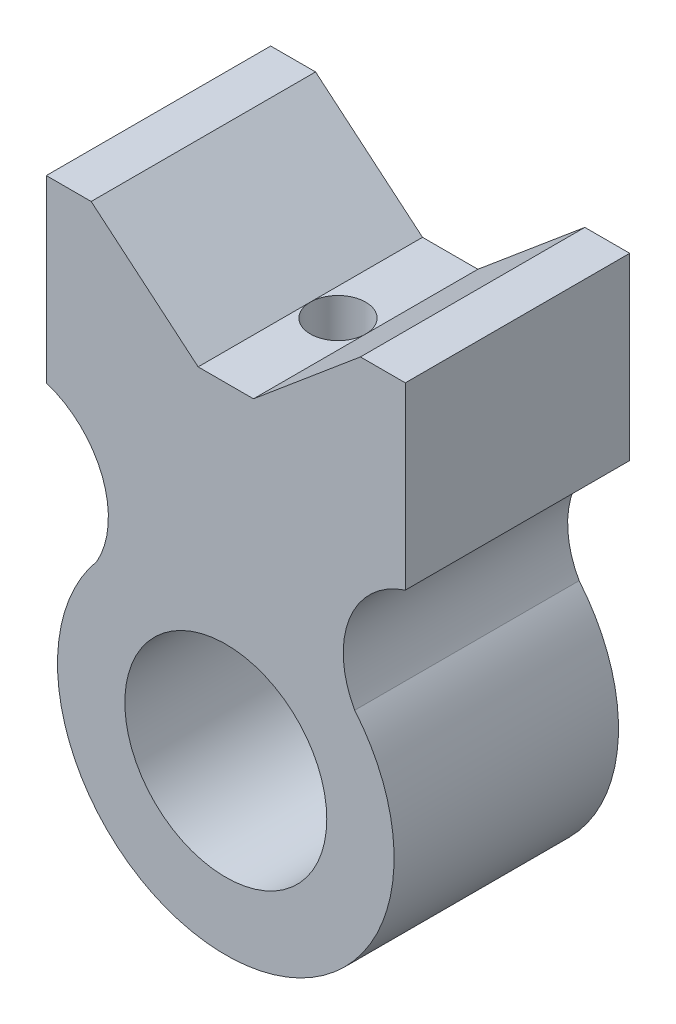
ISO-10303-21;
HEADER;
FILE_DESCRIPTION(('STEP AP214'),'2;1');
FILE_NAME('part.step','',(''),(''),'','','');
FILE_SCHEMA(('AUTOMOTIVE_DESIGN { 1 0 10303 214 1 1 1 1 }'));
ENDSEC;
DATA;
#1=APPLICATION_CONTEXT('core data for automotive mechanical design processes');
#2=APPLICATION_PROTOCOL_DEFINITION('international standard','automotive_design',2000,#1);
#3=PRODUCT_CONTEXT('',#1,'mechanical');
#4=PRODUCT('Part','Part','',(#3));
#5=PRODUCT_RELATED_PRODUCT_CATEGORY('part','',(#4));
#6=PRODUCT_DEFINITION_FORMATION('','',#4);
#7=PRODUCT_DEFINITION_CONTEXT('part definition',#1,'design');
#8=PRODUCT_DEFINITION('design','',#6,#7);
#9=PRODUCT_DEFINITION_SHAPE('','',#8);
#10=(LENGTH_UNIT() NAMED_UNIT(*) SI_UNIT(.MILLI.,.METRE.));
#11=(NAMED_UNIT(*) PLANE_ANGLE_UNIT() SI_UNIT($,.RADIAN.));
#12=(NAMED_UNIT(*) SI_UNIT($,.STERADIAN.) SOLID_ANGLE_UNIT());
#13=UNCERTAINTY_MEASURE_WITH_UNIT(LENGTH_MEASURE(1.E-05),#10,'distance_accuracy_value','');
#14=(GEOMETRIC_REPRESENTATION_CONTEXT(3) GLOBAL_UNCERTAINTY_ASSIGNED_CONTEXT((#13)) GLOBAL_UNIT_ASSIGNED_CONTEXT((#10,
#11,#12)) REPRESENTATION_CONTEXT('',''));
#15=CARTESIAN_POINT('',(0.,0.,0.));
#16=DIRECTION('',(0.,0.,1.));
#17=DIRECTION('',(1.,0.,0.));
#18=AXIS2_PLACEMENT_3D('',#15,#16,#17);
#19=CARTESIAN_POINT('',(46.1646162627975,33.8983044104148,25.));
#20=DIRECTION('',(0.,0.,-1.));
#21=DIRECTION('',(-1.,0.,0.));
#22=AXIS2_PLACEMENT_3D('',#19,#20,#21);
#23=PLANE('',#22);
#24=CARTESIAN_POINT('',(46.1646162627975,33.8983044104148,25.));
#25=DIRECTION('',(0.,0.,-1.));
#26=DIRECTION('',(-1.,0.,0.));
#27=AXIS2_PLACEMENT_3D('',#24,#25,#26);
#28=CIRCLE('',#27,20.);
#29=CARTESIAN_POINT('',(28.7266666169617,24.1045353632452,25.));
#30=VERTEX_POINT('',#29);
#31=CARTESIAN_POINT('',(39.9999281481161,52.9245131880117,25.));
#32=VERTEX_POINT('',#31);
#33=EDGE_CURVE('E185',#30,#32,#28,.T.);
#34=ORIENTED_EDGE('',*,*,#33,.T.);
#35=DIRECTION('',(0.,1.,0.));
#36=VECTOR('',#35,1.);
#37=CARTESIAN_POINT('',(39.9999281481161,92.9245131880117,25.));
#38=LINE('',#37,#36);
#39=CARTESIAN_POINT('',(39.9999281481161,92.9245131880117,25.));
#40=VERTEX_POINT('',#39);
#41=EDGE_CURVE('E111',#32,#40,#38,.T.);
#42=ORIENTED_EDGE('',*,*,#41,.T.);
#43=DIRECTION('',(-1.,0.,0.));
#44=VECTOR('',#43,1.);
#45=CARTESIAN_POINT('',(29.9999281481161,92.9245131880117,25.));
#46=LINE('',#45,#44);
#47=CARTESIAN_POINT('',(29.9999281481161,92.9245131880117,25.));
#48=VERTEX_POINT('',#47);
#49=EDGE_CURVE('E202',#40,#48,#46,.T.);
#50=ORIENTED_EDGE('',*,*,#49,.T.);
#51=DIRECTION('',(-0.766044443118979,-0.642787609686538,0.));
#52=VECTOR('',#51,1.);
#53=CARTESIAN_POINT('',(6.16485629623179,72.9245131880117,25.));
#54=LINE('',#53,#52);
#55=CARTESIAN_POINT('',(6.16485629623179,72.9245131880117,25.));
#56=VERTEX_POINT('',#55);
#57=EDGE_CURVE('E217',#48,#56,#54,.T.);
#58=ORIENTED_EDGE('',*,*,#57,.T.);
#59=DIRECTION('',(-1.,0.,0.));
#60=VECTOR('',#59,1.);
#61=CARTESIAN_POINT('',(-6.165,72.9245131880117,25.));
#62=LINE('',#61,#60);
#63=CARTESIAN_POINT('',(-6.165,72.9245131880117,25.));
#64=VERTEX_POINT('',#63);
#65=EDGE_CURVE('E219',#56,#64,#62,.T.);
#66=ORIENTED_EDGE('',*,*,#65,.T.);
#67=DIRECTION('',(-0.766044443118974,0.642787609686544,0.));
#68=VECTOR('',#67,1.);
#69=CARTESIAN_POINT('',(-30.0000718518839,92.9245131880117,25.));
#70=LINE('',#69,#68);
#71=CARTESIAN_POINT('',(-30.0000718518839,92.9245131880117,25.));
#72=VERTEX_POINT('',#71);
#73=EDGE_CURVE('E225',#64,#72,#70,.T.);
#74=ORIENTED_EDGE('',*,*,#73,.T.);
#75=DIRECTION('',(-1.,0.,0.));
#76=VECTOR('',#75,1.);
#77=CARTESIAN_POINT('',(-40.0000718518839,92.9245131880117,25.));
#78=LINE('',#77,#76);
#79=CARTESIAN_POINT('',(-40.0000718518839,92.9245131880117,25.));
#80=VERTEX_POINT('',#79);
#81=EDGE_CURVE('E140',#72,#80,#78,.T.);
#82=ORIENTED_EDGE('',*,*,#81,.T.);
#83=DIRECTION('',(0.,-1.,0.));
#84=VECTOR('',#83,1.);
#85=CARTESIAN_POINT('',(-40.0000718518839,52.9245131880117,25.));
#86=LINE('',#85,#84);
#87=CARTESIAN_POINT('',(-40.0000718518839,52.9245131880117,25.));
#88=VERTEX_POINT('',#87);
#89=EDGE_CURVE('E132',#80,#88,#86,.T.);
#90=ORIENTED_EDGE('',*,*,#89,.T.);
#91=CARTESIAN_POINT('',(-46.1646383870159,33.8982650178145,25.));
#92=DIRECTION('',(0.,0.,-1.));
#93=DIRECTION('',(1.,0.,0.));
#94=AXIS2_PLACEMENT_3D('',#91,#92,#93);
#95=CIRCLE('',#94,20.);
#96=CARTESIAN_POINT('',(-28.7266666169617,24.1045353632452,25.));
#97=VERTEX_POINT('',#96);
#98=EDGE_CURVE('E137',#88,#97,#95,.T.);
#99=ORIENTED_EDGE('',*,*,#98,.T.);
#100=CARTESIAN_POINT('',(0.,0.,25.));
#101=DIRECTION('',(0.,0.,1.));
#102=DIRECTION('',(1.,0.,0.));
#103=AXIS2_PLACEMENT_3D('',#100,#101,#102);
#104=CIRCLE('',#103,37.5);
#105=EDGE_CURVE('E69',#97,#30,#104,.T.);
#106=ORIENTED_EDGE('',*,*,#105,.T.);
#107=EDGE_LOOP('',(#34,#42,#50,#58,#66,#74,#82,#90,#99,#106));
#108=FACE_BOUND('',#107,.T.);
#109=CARTESIAN_POINT('',(0.,0.,25.));
#110=DIRECTION('',(0.,0.,1.));
#111=DIRECTION('',(1.,0.,0.));
#112=AXIS2_PLACEMENT_3D('',#109,#110,#111);
#113=CIRCLE('',#112,22.5);
#114=CARTESIAN_POINT('',(22.5,0.,25.));
#115=VERTEX_POINT('',#114);
#116=EDGE_CURVE('E164',#115,#115,#113,.T.);
#117=ORIENTED_EDGE('',*,*,#116,.F.);
#118=EDGE_LOOP('',(#117));
#119=FACE_BOUND('',#118,.T.);
#120=ADVANCED_FACE('F41',(#108,#119),#23,.F.);
#121=CARTESIAN_POINT('',(46.1646162627975,33.8983044104148,-25.));
#122=DIRECTION('',(0.,0.,-1.));
#123=DIRECTION('',(-1.,0.,0.));
#124=AXIS2_PLACEMENT_3D('',#121,#122,#123);
#125=PLANE('',#124);
#126=CARTESIAN_POINT('',(46.1646162627975,33.8983044104148,-25.));
#127=DIRECTION('',(0.,0.,-1.));
#128=DIRECTION('',(-1.,0.,0.));
#129=AXIS2_PLACEMENT_3D('',#126,#127,#128);
#130=CIRCLE('',#129,20.);
#131=CARTESIAN_POINT('',(28.7266666169617,24.1045353632452,-25.));
#132=VERTEX_POINT('',#131);
#133=CARTESIAN_POINT('',(39.9999281481161,52.9245131880117,-25.));
#134=VERTEX_POINT('',#133);
#135=EDGE_CURVE('E161',#132,#134,#130,.T.);
#136=ORIENTED_EDGE('',*,*,#135,.F.);
#137=CARTESIAN_POINT('',(0.,0.,-25.));
#138=DIRECTION('',(0.,0.,1.));
#139=DIRECTION('',(1.,0.,0.));
#140=AXIS2_PLACEMENT_3D('',#137,#138,#139);
#141=CIRCLE('',#140,37.5);
#142=CARTESIAN_POINT('',(-28.7266666169617,24.1045353632452,-25.));
#143=VERTEX_POINT('',#142);
#144=EDGE_CURVE('E106',#143,#132,#141,.T.);
#145=ORIENTED_EDGE('',*,*,#144,.F.);
#146=CARTESIAN_POINT('',(-46.1646383870159,33.8982650178145,-25.));
#147=DIRECTION('',(0.,0.,-1.));
#148=DIRECTION('',(1.,0.,0.));
#149=AXIS2_PLACEMENT_3D('',#146,#147,#148);
#150=CIRCLE('',#149,20.);
#151=CARTESIAN_POINT('',(-40.0000718518839,52.9245131880117,-25.));
#152=VERTEX_POINT('',#151);
#153=EDGE_CURVE('E178',#152,#143,#150,.T.);
#154=ORIENTED_EDGE('',*,*,#153,.F.);
#155=DIRECTION('',(0.,-1.,0.));
#156=VECTOR('',#155,1.);
#157=CARTESIAN_POINT('',(-40.0000718518839,52.9245131880117,-25.));
#158=LINE('',#157,#156);
#159=CARTESIAN_POINT('',(-40.0000718518839,92.9245131880117,-25.));
#160=VERTEX_POINT('',#159);
#161=EDGE_CURVE('E149',#160,#152,#158,.T.);
#162=ORIENTED_EDGE('',*,*,#161,.F.);
#163=DIRECTION('',(-1.,0.,0.));
#164=VECTOR('',#163,1.);
#165=CARTESIAN_POINT('',(-40.0000718518839,92.9245131880117,-25.));
#166=LINE('',#165,#164);
#167=CARTESIAN_POINT('',(-30.0000718518839,92.9245131880117,-25.));
#168=VERTEX_POINT('',#167);
#169=EDGE_CURVE('E176',#168,#160,#166,.T.);
#170=ORIENTED_EDGE('',*,*,#169,.F.);
#171=DIRECTION('',(-0.766044443118974,0.642787609686544,0.));
#172=VECTOR('',#171,1.);
#173=CARTESIAN_POINT('',(-30.0000718518839,92.9245131880117,-25.));
#174=LINE('',#173,#172);
#175=CARTESIAN_POINT('',(-6.165,72.9245131880117,-25.));
#176=VERTEX_POINT('',#175);
#177=EDGE_CURVE('E173',#176,#168,#174,.T.);
#178=ORIENTED_EDGE('',*,*,#177,.F.);
#179=DIRECTION('',(-1.,0.,0.));
#180=VECTOR('',#179,1.);
#181=CARTESIAN_POINT('',(-6.165,72.9245131880117,-25.));
#182=LINE('',#181,#180);
#183=CARTESIAN_POINT('',(6.16485629623179,72.9245131880117,-25.));
#184=VERTEX_POINT('',#183);
#185=EDGE_CURVE('E175',#184,#176,#182,.T.);
#186=ORIENTED_EDGE('',*,*,#185,.F.);
#187=DIRECTION('',(-0.766044443118979,-0.642787609686538,0.));
#188=VECTOR('',#187,1.);
#189=CARTESIAN_POINT('',(6.16485629623179,72.9245131880117,-25.));
#190=LINE('',#189,#188);
#191=CARTESIAN_POINT('',(29.9999281481161,92.9245131880117,-25.));
#192=VERTEX_POINT('',#191);
#193=EDGE_CURVE('E166',#192,#184,#190,.T.);
#194=ORIENTED_EDGE('',*,*,#193,.F.);
#195=DIRECTION('',(-1.,0.,0.));
#196=VECTOR('',#195,1.);
#197=CARTESIAN_POINT('',(29.9999281481161,92.9245131880117,-25.));
#198=LINE('',#197,#196);
#199=CARTESIAN_POINT('',(39.9999281481161,92.9245131880117,-25.));
#200=VERTEX_POINT('',#199);
#201=EDGE_CURVE('E170',#200,#192,#198,.T.);
#202=ORIENTED_EDGE('',*,*,#201,.F.);
#203=DIRECTION('',(0.,1.,0.));
#204=VECTOR('',#203,1.);
#205=CARTESIAN_POINT('',(39.9999281481161,92.9245131880117,-25.));
#206=LINE('',#205,#204);
#207=EDGE_CURVE('E163',#134,#200,#206,.T.);
#208=ORIENTED_EDGE('',*,*,#207,.F.);
#209=EDGE_LOOP('',(#136,#145,#154,#162,#170,#178,#186,#194,#202,#208));
#210=FACE_BOUND('',#209,.T.);
#211=CARTESIAN_POINT('',(0.,0.,-25.));
#212=DIRECTION('',(0.,0.,1.));
#213=DIRECTION('',(1.,0.,0.));
#214=AXIS2_PLACEMENT_3D('',#211,#212,#213);
#215=CIRCLE('',#214,22.5);
#216=CARTESIAN_POINT('',(22.5,0.,-25.));
#217=VERTEX_POINT('',#216);
#218=EDGE_CURVE('E241',#217,#217,#215,.T.);
#219=ORIENTED_EDGE('',*,*,#218,.T.);
#220=EDGE_LOOP('',(#219));
#221=FACE_BOUND('',#220,.T.);
#222=ADVANCED_FACE('F207',(#210,#221),#125,.T.);
#223=CARTESIAN_POINT('',(46.1646162627975,33.8983044104148,25.));
#224=DIRECTION('',(0.,0.,-1.));
#225=DIRECTION('',(-1.,0.,0.));
#226=AXIS2_PLACEMENT_3D('',#223,#224,#225);
#227=CYLINDRICAL_SURFACE('',#226,20.);
#228=ORIENTED_EDGE('',*,*,#135,.T.);
#229=DIRECTION('',(0.,0.,-1.));
#230=VECTOR('',#229,1.);
#231=CARTESIAN_POINT('',(39.9999281481161,52.9245131880117,25.));
#232=LINE('',#231,#230);
#233=EDGE_CURVE('E11',#32,#134,#232,.T.);
#234=ORIENTED_EDGE('',*,*,#233,.F.);
#235=ORIENTED_EDGE('',*,*,#33,.F.);
#236=DIRECTION('',(0.,0.,-1.));
#237=VECTOR('',#236,1.);
#238=CARTESIAN_POINT('',(28.7266666169617,24.1045353632452,25.));
#239=LINE('',#238,#237);
#240=EDGE_CURVE('E160',#30,#132,#239,.T.);
#241=ORIENTED_EDGE('',*,*,#240,.T.);
#242=EDGE_LOOP('',(#228,#234,#235,#241));
#243=FACE_BOUND('',#242,.T.);
#244=ADVANCED_FACE('F43',(#243),#227,.F.);
#245=CARTESIAN_POINT('',(39.9999281481161,92.9245131880117,25.));
#246=DIRECTION('',(-1.,0.,0.));
#247=DIRECTION('',(0.,0.,1.));
#248=AXIS2_PLACEMENT_3D('',#245,#246,#247);
#249=PLANE('',#248);
#250=ORIENTED_EDGE('',*,*,#207,.T.);
#251=DIRECTION('',(0.,0.,-1.));
#252=VECTOR('',#251,1.);
#253=CARTESIAN_POINT('',(39.9999281481161,92.9245131880117,25.));
#254=LINE('',#253,#252);
#255=EDGE_CURVE('E54',#40,#200,#254,.T.);
#256=ORIENTED_EDGE('',*,*,#255,.F.);
#257=ORIENTED_EDGE('',*,*,#41,.F.);
#258=ORIENTED_EDGE('',*,*,#233,.T.);
#259=EDGE_LOOP('',(#250,#256,#257,#258));
#260=FACE_BOUND('',#259,.T.);
#261=ADVANCED_FACE('F263',(#260),#249,.F.);
#262=CARTESIAN_POINT('',(29.9999281481161,92.9245131880117,25.));
#263=DIRECTION('',(0.,-1.,0.));
#264=DIRECTION('',(0.,0.,-1.));
#265=AXIS2_PLACEMENT_3D('',#262,#263,#264);
#266=PLANE('',#265);
#267=ORIENTED_EDGE('',*,*,#201,.T.);
#268=DIRECTION('',(0.,0.,-1.));
#269=VECTOR('',#268,1.);
#270=CARTESIAN_POINT('',(29.9999281481161,92.9245131880117,25.));
#271=LINE('',#270,#269);
#272=EDGE_CURVE('E198',#48,#192,#271,.T.);
#273=ORIENTED_EDGE('',*,*,#272,.F.);
#274=ORIENTED_EDGE('',*,*,#49,.F.);
#275=ORIENTED_EDGE('',*,*,#255,.T.);
#276=EDGE_LOOP('',(#267,#273,#274,#275));
#277=FACE_BOUND('',#276,.T.);
#278=ADVANCED_FACE('F201',(#277),#266,.F.);
#279=CARTESIAN_POINT('',(6.16485629623179,72.9245131880117,25.));
#280=DIRECTION('',(0.642787609686538,-0.766044443118979,0.));
#281=DIRECTION('',(0.766044443118979,0.642787609686538,0.));
#282=AXIS2_PLACEMENT_3D('',#279,#280,#281);
#283=PLANE('',#282);
#284=ORIENTED_EDGE('',*,*,#193,.T.);
#285=DIRECTION('',(0.,0.,-1.));
#286=VECTOR('',#285,1.);
#287=CARTESIAN_POINT('',(6.16485629623179,72.9245131880117,25.));
#288=LINE('',#287,#286);
#289=CARTESIAN_POINT('',(6.16485629623179,72.9245131880117,0.));
#290=VERTEX_POINT('',#289);
#291=EDGE_CURVE('E192',#290,#184,#288,.T.);
#292=ORIENTED_EDGE('',*,*,#291,.F.);
#293=EDGE_CURVE('E194',#56,#290,#288,.T.);
#294=ORIENTED_EDGE('',*,*,#293,.F.);
#295=ORIENTED_EDGE('',*,*,#57,.F.);
#296=ORIENTED_EDGE('',*,*,#272,.T.);
#297=EDGE_LOOP('',(#284,#292,#294,#295,#296));
#298=FACE_BOUND('',#297,.T.);
#299=ADVANCED_FACE('F214',(#298),#283,.F.);
#300=CARTESIAN_POINT('',(-6.165,72.9245131880117,25.));
#301=DIRECTION('',(0.,-1.,0.));
#302=DIRECTION('',(0.,0.,-1.));
#303=AXIS2_PLACEMENT_3D('',#300,#301,#302);
#304=PLANE('',#303);
#305=ORIENTED_EDGE('',*,*,#293,.T.);
#306=CARTESIAN_POINT('',(0.,72.9245131880117,0.));
#307=DIRECTION('',(0.,1.,0.));
#308=DIRECTION('',(0.,0.,1.));
#309=AXIS2_PLACEMENT_3D('',#306,#307,#308);
#310=CIRCLE('',#309,6.16485629623179);
#311=EDGE_CURVE('E58',#290,#290,#310,.T.);
#312=ORIENTED_EDGE('',*,*,#311,.F.);
#313=ORIENTED_EDGE('',*,*,#291,.T.);
#314=ORIENTED_EDGE('',*,*,#185,.T.);
#315=DIRECTION('',(0.,0.,-1.));
#316=VECTOR('',#315,1.);
#317=CARTESIAN_POINT('',(-6.165,72.9245131880117,25.));
#318=LINE('',#317,#316);
#319=EDGE_CURVE('E188',#64,#176,#318,.T.);
#320=ORIENTED_EDGE('',*,*,#319,.F.);
#321=ORIENTED_EDGE('',*,*,#65,.F.);
#322=EDGE_LOOP('',(#305,#312,#313,#314,#320,#321));
#323=FACE_BOUND('',#322,.T.);
#324=ADVANCED_FACE('F277',(#323),#304,.F.);
#325=CARTESIAN_POINT('',(-30.0000718518839,92.9245131880117,25.));
#326=DIRECTION('',(-0.642787609686544,-0.766044443118974,0.));
#327=DIRECTION('',(0.766044443118974,-0.642787609686544,0.));
#328=AXIS2_PLACEMENT_3D('',#325,#326,#327);
#329=PLANE('',#328);
#330=ORIENTED_EDGE('',*,*,#177,.T.);
#331=DIRECTION('',(0.,0.,-1.));
#332=VECTOR('',#331,1.);
#333=CARTESIAN_POINT('',(-30.0000718518839,92.9245131880117,25.));
#334=LINE('',#333,#332);
#335=EDGE_CURVE('E186',#72,#168,#334,.T.);
#336=ORIENTED_EDGE('',*,*,#335,.F.);
#337=ORIENTED_EDGE('',*,*,#73,.F.);
#338=ORIENTED_EDGE('',*,*,#319,.T.);
#339=EDGE_LOOP('',(#330,#336,#337,#338));
#340=FACE_BOUND('',#339,.T.);
#341=ADVANCED_FACE('F231',(#340),#329,.F.);
#342=CARTESIAN_POINT('',(-40.0000718518839,92.9245131880117,25.));
#343=DIRECTION('',(0.,-1.,0.));
#344=DIRECTION('',(0.,0.,-1.));
#345=AXIS2_PLACEMENT_3D('',#342,#343,#344);
#346=PLANE('',#345);
#347=ORIENTED_EDGE('',*,*,#169,.T.);
#348=DIRECTION('',(0.,0.,-1.));
#349=VECTOR('',#348,1.);
#350=CARTESIAN_POINT('',(-40.0000718518839,92.9245131880117,25.));
#351=LINE('',#350,#349);
#352=EDGE_CURVE('E155',#80,#160,#351,.T.);
#353=ORIENTED_EDGE('',*,*,#352,.F.);
#354=ORIENTED_EDGE('',*,*,#81,.F.);
#355=ORIENTED_EDGE('',*,*,#335,.T.);
#356=EDGE_LOOP('',(#347,#353,#354,#355));
#357=FACE_BOUND('',#356,.T.);
#358=ADVANCED_FACE('F233',(#357),#346,.F.);
#359=CARTESIAN_POINT('',(-40.0000718518839,52.9245131880117,25.));
#360=DIRECTION('',(1.,0.,0.));
#361=DIRECTION('',(0.,1.,0.));
#362=AXIS2_PLACEMENT_3D('',#359,#360,#361);
#363=PLANE('',#362);
#364=ORIENTED_EDGE('',*,*,#161,.T.);
#365=DIRECTION('',(0.,0.,-1.));
#366=VECTOR('',#365,1.);
#367=CARTESIAN_POINT('',(-40.0000718518839,52.9245131880117,25.));
#368=LINE('',#367,#366);
#369=EDGE_CURVE('E148',#88,#152,#368,.T.);
#370=ORIENTED_EDGE('',*,*,#369,.F.);
#371=ORIENTED_EDGE('',*,*,#89,.F.);
#372=ORIENTED_EDGE('',*,*,#352,.T.);
#373=EDGE_LOOP('',(#364,#370,#371,#372));
#374=FACE_BOUND('',#373,.T.);
#375=ADVANCED_FACE('F150',(#374),#363,.F.);
#376=CARTESIAN_POINT('',(-46.1646383870159,33.8982650178145,25.));
#377=DIRECTION('',(0.,0.,-1.));
#378=DIRECTION('',(-1.,0.,0.));
#379=AXIS2_PLACEMENT_3D('',#376,#377,#378);
#380=CYLINDRICAL_SURFACE('',#379,20.);
#381=ORIENTED_EDGE('',*,*,#153,.T.);
#382=DIRECTION('',(0.,0.,-1.));
#383=VECTOR('',#382,1.);
#384=CARTESIAN_POINT('',(-28.7266666169617,24.1045353632452,25.));
#385=LINE('',#384,#383);
#386=EDGE_CURVE('E153',#97,#143,#385,.T.);
#387=ORIENTED_EDGE('',*,*,#386,.F.);
#388=ORIENTED_EDGE('',*,*,#98,.F.);
#389=ORIENTED_EDGE('',*,*,#369,.T.);
#390=EDGE_LOOP('',(#381,#387,#388,#389));
#391=FACE_BOUND('',#390,.T.);
#392=ADVANCED_FACE('F154',(#391),#380,.F.);
#393=CARTESIAN_POINT('',(0.,0.,25.));
#394=DIRECTION('',(0.,0.,-1.));
#395=DIRECTION('',(-1.,0.,0.));
#396=AXIS2_PLACEMENT_3D('',#393,#394,#395);
#397=CYLINDRICAL_SURFACE('',#396,37.5);
#398=ORIENTED_EDGE('',*,*,#144,.T.);
#399=ORIENTED_EDGE('',*,*,#240,.F.);
#400=ORIENTED_EDGE('',*,*,#105,.F.);
#401=ORIENTED_EDGE('',*,*,#386,.T.);
#402=EDGE_LOOP('',(#398,#399,#400,#401));
#403=FACE_BOUND('',#402,.T.);
#404=ADVANCED_FACE('F235',(#403),#397,.T.);
#405=CARTESIAN_POINT('',(0.,0.,25.));
#406=DIRECTION('',(0.,0.,-1.));
#407=DIRECTION('',(-1.,0.,0.));
#408=AXIS2_PLACEMENT_3D('',#405,#406,#407);
#409=CYLINDRICAL_SURFACE('',#408,22.5);
#410=CARTESIAN_POINT('',(0.,22.5,6.16485629623179));
#411=CARTESIAN_POINT('',(-0.169804680899999,22.5000039958812,6.16486247325919));
#412=CARTESIAN_POINT('',(-0.339546424729067,22.4980751875444,6.1578400967572));
#413=CARTESIAN_POINT('',(-0.677833671554656,22.4904226505744,6.12982649815303));
#414=CARTESIAN_POINT('',(-0.846379074070752,22.4846986069047,6.10883411642172));
#415=CARTESIAN_POINT('',(-1.18102844003461,22.4696072914284,6.05305025199593));
#416=CARTESIAN_POINT('',(-1.34713191358289,22.4602392986512,6.01825603852442));
#417=CARTESIAN_POINT('',(-1.67575672869155,22.438114170694,5.93515171287779));
#418=CARTESIAN_POINT('',(-1.83827672420854,22.4253557847171,5.88683661217529));
#419=CARTESIAN_POINT('',(-2.15827076515482,22.3968218534693,5.77718588696579));
#420=CARTESIAN_POINT('',(-2.3157530429585,22.3810515587545,5.71587290105962));
#421=CARTESIAN_POINT('',(-2.62497388925292,22.3468951568018,5.5806323107831));
#422=CARTESIAN_POINT('',(-2.77671030869297,22.3285080828419,5.50670004242407));
#423=CARTESIAN_POINT('',(-3.07336281608163,22.2896120529047,5.34679971837364));
#424=CARTESIAN_POINT('',(-3.21828109515303,22.2691037854791,5.2608355651203));
#425=CARTESIAN_POINT('',(-3.50046321085769,22.2264968395459,5.07745673060431));
#426=CARTESIAN_POINT('',(-3.63772408920782,22.2043975538295,4.98003766852128));
#427=CARTESIAN_POINT('',(-4.04242418801313,22.1355944763658,4.66712137170301));
#428=CARTESIAN_POINT('',(-4.29651941441901,22.0872414681114,4.43433730935693));
#429=CARTESIAN_POINT('',(-4.76254061121995,21.9914771105941,3.92958784969431));
#430=CARTESIAN_POINT('',(-4.97446082637198,21.9440658906419,3.65761711364424));
#431=CARTESIAN_POINT('',(-5.2580980806478,21.8772043304826,3.22313853618599));
#432=CARTESIAN_POINT('',(-5.34761238075598,21.8554421449833,3.07234116943093));
#433=CARTESIAN_POINT('',(-5.51357225610034,21.8141659169717,2.76345191537595));
#434=CARTESIAN_POINT('',(-5.5900229574015,21.794650993634,2.60536292032679));
#435=CARTESIAN_POINT('',(-5.72927110151088,21.7584612029785,2.28292866551506));
#436=CARTESIAN_POINT('',(-5.79206512294058,21.7417870475782,2.11858185008447));
#437=CARTESIAN_POINT('',(-5.90342876265715,21.7118137557504,1.78490830560441));
#438=CARTESIAN_POINT('',(-5.95200443064792,21.698513184234,1.61558372836645));
#439=CARTESIAN_POINT('',(-6.03356495191446,21.6759738733472,1.27715822763984));
#440=CARTESIAN_POINT('',(-6.06688752860178,21.6666475000157,1.10814449512105));
#441=CARTESIAN_POINT('',(-6.1192758652691,21.651909975297,0.767817753111401));
#442=CARTESIAN_POINT('',(-6.1383472429228,21.6464972812056,0.596505676740326));
#443=CARTESIAN_POINT('',(-6.16207907593207,21.6397535656216,0.252802858011335));
#444=CARTESIAN_POINT('',(-6.16673927908287,21.6384226155623,0.0804120968286499));
#445=CARTESIAN_POINT('',(-6.16160442899097,21.6398853621992,-0.264134791115567));
#446=CARTESIAN_POINT('',(-6.15180962548001,21.6426789876373,-0.436290921879257));
#447=CARTESIAN_POINT('',(-6.11836340017467,21.6521573608376,-0.773953973975949));
#448=CARTESIAN_POINT('',(-6.0951334973235,21.6587237022174,-0.939506186833977));
#449=CARTESIAN_POINT('',(-6.03534349457947,21.6754605863186,-1.26805820967563));
#450=CARTESIAN_POINT('',(-5.99877883862963,21.6856323608675,-1.43105712740451));
#451=CARTESIAN_POINT('',(-5.91263696490615,21.7092771742066,-1.75327736663293));
#452=CARTESIAN_POINT('',(-5.86306371131661,21.7227492072074,-1.9124998228651));
#453=CARTESIAN_POINT('',(-5.75127143603937,21.7526141505211,-2.22622361587916));
#454=CARTESIAN_POINT('',(-5.68904764295528,21.7690081626266,-2.38072314594991));
#455=CARTESIAN_POINT('',(-5.55165226206705,21.8044547044247,-2.68568404968862));
#456=CARTESIAN_POINT('',(-5.47634092667827,21.8235354560967,-2.8360791591441));
#457=CARTESIAN_POINT('',(-5.31378844542516,21.8636835917447,-3.13006873968286));
#458=CARTESIAN_POINT('',(-5.22654294287635,21.8847517003489,-3.27366070131716));
#459=CARTESIAN_POINT('',(-5.04075809432739,21.9282889318972,-3.55307658857817));
#460=CARTESIAN_POINT('',(-4.94222084369121,21.9507577945573,-3.68890194843213));
#461=CARTESIAN_POINT('',(-4.73444381489767,21.996507889281,-3.95203868102209));
#462=CARTESIAN_POINT('',(-4.62520002397133,22.0197894238097,-4.07934683122971));
#463=CARTESIAN_POINT('',(-4.3928153783924,22.0673449103641,-4.32881845856397));
#464=CARTESIAN_POINT('',(-4.26932711240318,22.0916255806708,-4.45065728217631));
#465=CARTESIAN_POINT('',(-4.01242719594079,22.1397269373919,-4.68358369306341));
#466=CARTESIAN_POINT('',(-3.87901181524925,22.1635474466177,-4.7946672024659));
#467=CARTESIAN_POINT('',(-3.60320531369759,22.2100531155921,-5.00524297323135));
#468=CARTESIAN_POINT('',(-3.46081698042209,22.2327386240555,-5.10473880739106));
#469=CARTESIAN_POINT('',(-3.16790460329755,22.276362132604,-5.29150391687559));
#470=CARTESIAN_POINT('',(-3.01737761548788,22.2972994932767,-5.3787687263638));
#471=CARTESIAN_POINT('',(-2.70852236690333,22.3369258262456,-5.54074969931487));
#472=CARTESIAN_POINT('',(-2.55016105092076,22.3556038778171,-5.61540555359664));
#473=CARTESIAN_POINT('',(-2.22739079163058,22.3900662858194,-5.75107195724721));
#474=CARTESIAN_POINT('',(-2.06298188252292,22.4058506586112,-5.81208258376781));
#475=CARTESIAN_POINT('',(-1.72933181798131,22.434068574467,-5.9199321371731));
#476=CARTESIAN_POINT('',(-1.56009159979869,22.4465027626309,-5.96677379259911));
#477=CARTESIAN_POINT('',(-1.21800814007337,22.4676616160537,-6.04588513238973));
#478=CARTESIAN_POINT('',(-1.04516492653661,22.4763863101352,-6.07815492997668));
#479=CARTESIAN_POINT('',(-0.702494113332748,22.489664391513,-6.12707054612797));
#480=CARTESIAN_POINT('',(-0.532734529600064,22.4943365020489,-6.14416143062089));
#481=CARTESIAN_POINT('',(-0.192321860947291,22.4998219324708,-6.16421400415301));
#482=CARTESIAN_POINT('',(-0.0216687938227659,22.5006353289206,-6.16717597353509));
#483=CARTESIAN_POINT('',(0.319253617813562,22.4983806966859,-6.15894490391073));
#484=CARTESIAN_POINT('',(0.489522995405853,22.4953130165286,-6.14775313593401));
#485=CARTESIAN_POINT('',(0.828434694697325,22.4853827042707,-6.11131698132565));
#486=CARTESIAN_POINT('',(0.9970770588896,22.4785201715556,-6.08607296271623));
#487=CARTESIAN_POINT('',(1.32844540846224,22.4613502610591,-6.02234425567868));
#488=CARTESIAN_POINT('',(1.49122318081215,22.45110830919,-5.98411065910267));
#489=CARTESIAN_POINT('',(1.81291973942967,22.4274237474967,-5.8946288436972));
#490=CARTESIAN_POINT('',(1.97183854648799,22.4139811549207,-5.84338069500246));
#491=CARTESIAN_POINT('',(2.28480146875957,22.3842444326981,-5.72825827258206));
#492=CARTESIAN_POINT('',(2.43884436991432,22.3679495993615,-5.66438088253093));
#493=CARTESIAN_POINT('',(2.74097580275037,22.332939239445,-5.52450983968426));
#494=CARTESIAN_POINT('',(2.88906624455624,22.3142244976675,-5.44852011319913));
#495=CARTESIAN_POINT('',(3.18142817982216,22.2744411772748,-5.28325149795397));
#496=CARTESIAN_POINT('',(3.32555686637158,22.2533318458392,-5.19372977935507));
#497=CARTESIAN_POINT('',(3.60575192136055,22.2096522925334,-5.00326836245644));
#498=CARTESIAN_POINT('',(3.74182093737019,22.1870825555557,-4.90233244572944));
#499=CARTESIAN_POINT('',(4.00517737836928,22.1410576842029,-4.68963449108057));
#500=CARTESIAN_POINT('',(4.1324600901976,22.1176020849097,-4.57786671881458));
#501=CARTESIAN_POINT('',(4.37733422616389,22.0704438177248,-4.34430864981719));
#502=CARTESIAN_POINT('',(4.49492895235705,22.0467412371433,-4.22252179651418));
#503=CARTESIAN_POINT('',(4.72315093123138,21.998996531183,-3.96581393645261));
#504=CARTESIAN_POINT('',(4.83345888623743,21.9749658958774,-3.83060668608148));
#505=CARTESIAN_POINT('',(5.04226249855185,21.9279967277358,-3.55125891460085));
#506=CARTESIAN_POINT('',(5.14076242945477,21.9050578016087,-3.40712165428925));
#507=CARTESIAN_POINT('',(5.32532660547586,21.8609219128613,-3.1107608952243));
#508=CARTESIAN_POINT('',(5.41138619991812,21.8397256029683,-2.95853440133937));
#509=CARTESIAN_POINT('',(5.57034093664364,21.7997252311009,-2.64713074356827));
#510=CARTESIAN_POINT('',(5.64324143179868,21.7809201973248,-2.48795643878912));
#511=CARTESIAN_POINT('',(5.7749832104623,21.7463602841155,-2.16456540495367));
#512=CARTESIAN_POINT('',(5.83389716983256,21.7305897220794,-2.00037997827362));
#513=CARTESIAN_POINT('',(5.93764476536082,21.7024714234429,-1.66740042498792));
#514=CARTESIAN_POINT('',(5.98248391766424,21.6901223461305,-1.49860813215013));
#515=CARTESIAN_POINT('',(6.05771300707976,21.6692325615847,-1.15760545606194));
#516=CARTESIAN_POINT('',(6.088103424471,21.6606917277651,-0.985395186624089));
#517=CARTESIAN_POINT('',(6.1341546058956,21.6476955504674,-0.638865030225768));
#518=CARTESIAN_POINT('',(6.14981581484355,21.6432400835857,-0.464545207148174));
#519=CARTESIAN_POINT('',(6.1659747695676,21.6386418367261,-0.121246495517261));
#520=CARTESIAN_POINT('',(6.16698223666735,21.6383540868257,0.0477066661779305));
#521=CARTESIAN_POINT('',(6.15513006104714,21.6417284977583,0.385145661860286));
#522=CARTESIAN_POINT('',(6.1422656550141,21.6453920153746,0.553631315391866));
#523=CARTESIAN_POINT('',(6.10278442610616,21.6565565379228,0.888783717584269));
#524=CARTESIAN_POINT('',(6.07617314196419,21.6640559973096,1.0554511712177));
#525=CARTESIAN_POINT('',(6.00941998585004,21.6826675092392,1.3859114331253));
#526=CARTESIAN_POINT('',(5.96927306955882,21.6937809085328,1.5497031457216));
#527=CARTESIAN_POINT('',(5.87620933504042,21.7191727672707,1.87175290266535));
#528=CARTESIAN_POINT('',(5.82341086684375,21.7334217988357,2.03004751525733));
#529=CARTESIAN_POINT('',(5.70525295384199,21.7647380531881,2.34164816560734));
#530=CARTESIAN_POINT('',(5.63988923454852,21.7818062347243,2.49495248493917));
#531=CARTESIAN_POINT('',(5.49710117428335,21.8182791405506,2.79553494504101));
#532=CARTESIAN_POINT('',(5.41967746329449,21.8376837427802,2.94281340007948));
#533=CARTESIAN_POINT('',(5.25330756182772,21.8783017849108,3.23045180290698));
#534=CARTESIAN_POINT('',(5.16436099106973,21.8995152845015,3.37081152215114));
#535=CARTESIAN_POINT('',(4.97259584723247,21.9438663704224,3.64801639040249));
#536=CARTESIAN_POINT('',(4.86943180493722,21.9670432837367,3.78461636152603));
#537=CARTESIAN_POINT('',(4.65220770643028,22.0140706291764,4.04865840898731));
#538=CARTESIAN_POINT('',(4.53815104960987,22.0379208495484,4.17610332084142));
#539=CARTESIAN_POINT('',(4.29978140862809,22.0856663784239,4.42114987337088));
#540=CARTESIAN_POINT('',(4.17546249973118,22.1095617050799,4.53874574783113));
#541=CARTESIAN_POINT('',(3.91746164412659,22.156729971619,4.76321057423879));
#542=CARTESIAN_POINT('',(3.78378307773561,22.180003132049,4.87008336533246));
#543=CARTESIAN_POINT('',(3.50463256043331,22.2258411665092,5.0748060751261));
#544=CARTESIAN_POINT('',(3.35895785284907,22.2483767269151,5.17238636844375));
#545=CARTESIAN_POINT('',(3.05967231348559,22.2915063756556,5.35486395641765));
#546=CARTESIAN_POINT('',(2.90606441667362,22.3121011741427,5.43976589696433));
#547=CARTESIAN_POINT('',(2.59195233153521,22.3507672062143,5.5962489844445));
#548=CARTESIAN_POINT('',(2.43145042709296,22.3688392672405,5.66783450165363));
#549=CARTESIAN_POINT('',(2.10470072849753,22.4019473316377,5.79711841145669));
#550=CARTESIAN_POINT('',(1.93845366424099,22.4169837190286,5.85481856076054));
#551=CARTESIAN_POINT('',(1.48388924444167,22.4528414203248,5.99103699620327));
#552=CARTESIAN_POINT('',(1.19114960421748,22.4704043592258,6.05609061956663));
#553=CARTESIAN_POINT('',(0.59887427527355,22.4939794853905,6.1429924250602));
#554=CARTESIAN_POINT('',(0.299339345299876,22.4999929558805,6.16484540708947));
#555=CARTESIAN_POINT('',(0.,22.5,6.16485629623179));
#556=B_SPLINE_CURVE_WITH_KNOTS('',3,(#410,#411,#412,#413,#414,#415,#416,#417,#418,#419,#420,
#421,#422,#423,#424,#425,#426,#427,#428,#429,#430,#431,#432,#433,#434,#435,#436,#437,#438,#439,
#440,#441,#442,#443,#444,#445,#446,#447,#448,#449,#450,#451,#452,#453,#454,#455,#456,#457,#458,
#459,#460,#461,#462,#463,#464,#465,#466,#467,#468,#469,#470,#471,#472,#473,#474,#475,#476,#477,
#478,#479,#480,#481,#482,#483,#484,#485,#486,#487,#488,#489,#490,#491,#492,#493,#494,#495,#496,
#497,#498,#499,#500,#501,#502,#503,#504,#505,#506,#507,#508,#509,#510,#511,#512,#513,#514,#515,
#516,#517,#518,#519,#520,#521,#522,#523,#524,#525,#526,#527,#528,#529,#530,#531,#532,#533,#534,
#535,#536,#537,#538,#539,#540,#541,#542,#543,#544,#545,#546,#547,#548,#549,#550,#551,#552,#553,
#554,#555),.UNSPECIFIED.,.T.,.F.,(4,2,2,2,2,2,2,2,2,2,2,2,2,2,2,2,2,2,2,2,2,2,2,2,2,2,2,2,2,2,2,
2,2,2,2,2,2,2,2,2,2,2,2,2,2,2,2,2,2,2,2,2,2,2,2,2,2,2,2,2,2,2,2,2,2,2,2,2,2,2,2,2,4),(0.,
0.50914972010305,1.01834170923154,1.52763449540914,2.03711543330446,2.54571618642288,
3.05450532307149,3.56312981912047,4.0719494703192,5.11081849206933,6.149829181836,
6.67941310026188,7.20878873406599,7.73829683881884,8.2675793169291,8.78449659551014,
9.30121000305823,9.81793245336963,10.3346459766367,10.8359652462999,11.3374559613799,
11.8387940314493,12.3403215428645,12.8475764450296,13.355017022235,13.8623635877667,
14.3699010373049,14.8947889752192,15.4198751511624,15.9447989976672,16.4699140097681,
16.9974736008746,17.5250302090189,18.0524851599765,18.5799360125748,19.0913554700863,
19.6027647800813,20.1141281679107,20.6254781639894,21.1274584115945,21.6294359541121,
22.1315375169197,22.6334766492726,23.1458210189722,23.6579961413548,24.1704439040787,
24.6827162750869,25.2105185192743,25.738129159296,26.2659365331708,26.7935287187942,
27.3183163335751,27.8428980180304,28.3674622640555,28.8920106644383,29.3982675367973,
29.9046983026239,30.4109251821929,30.9173409260597,31.4191925849084,31.921215268384,
32.4232117362792,32.9252247754004,33.4428552336585,33.9603246732903,34.4780949829921,
34.9956792508054,35.5253739166177,36.0548740008191,36.5842000022617,37.1134590006778,
38.0111108179088,38.9086628940204),.UNSPECIFIED.);
#557=CARTESIAN_POINT('',(0.,22.5,6.16485629623179));
#558=VERTEX_POINT('',#557);
#559=EDGE_CURVE('E44',#558,#558,#556,.T.);
#560=ORIENTED_EDGE('',*,*,#559,.F.);
#561=EDGE_LOOP('',(#560));
#562=FACE_BOUND('',#561,.T.);
#563=ORIENTED_EDGE('',*,*,#116,.T.);
#564=EDGE_LOOP('',(#563));
#565=FACE_BOUND('',#564,.T.);
#566=ORIENTED_EDGE('',*,*,#218,.F.);
#567=EDGE_LOOP('',(#566));
#568=FACE_BOUND('',#567,.T.);
#569=ADVANCED_FACE('F253',(#562,#565,#568),#409,.F.);
#570=CARTESIAN_POINT('',(0.,12.9245131880117,0.));
#571=DIRECTION('',(0.,1.,0.));
#572=DIRECTION('',(0.,0.,1.));
#573=AXIS2_PLACEMENT_3D('',#570,#571,#572);
#574=CYLINDRICAL_SURFACE('',#573,6.16485629623179);
#575=ORIENTED_EDGE('',*,*,#559,.T.);
#576=EDGE_LOOP('',(#575));
#577=FACE_BOUND('',#576,.T.);
#578=ORIENTED_EDGE('',*,*,#311,.T.);
#579=EDGE_LOOP('',(#578));
#580=FACE_BOUND('',#579,.T.);
#581=ADVANCED_FACE('F248',(#577,#580),#574,.F.);
#582=CLOSED_SHELL('',(#120,#222,#244,#261,#278,#299,#324,#341,#358,#375,#392,#404,#569,#581));
#583=MANIFOLD_SOLID_BREP('B2',#582);
#584=ADVANCED_BREP_SHAPE_REPRESENTATION('',(#18,#583),#14);
#585=SHAPE_DEFINITION_REPRESENTATION(#9,#584);
ENDSEC;
END-ISO-10303-21;
